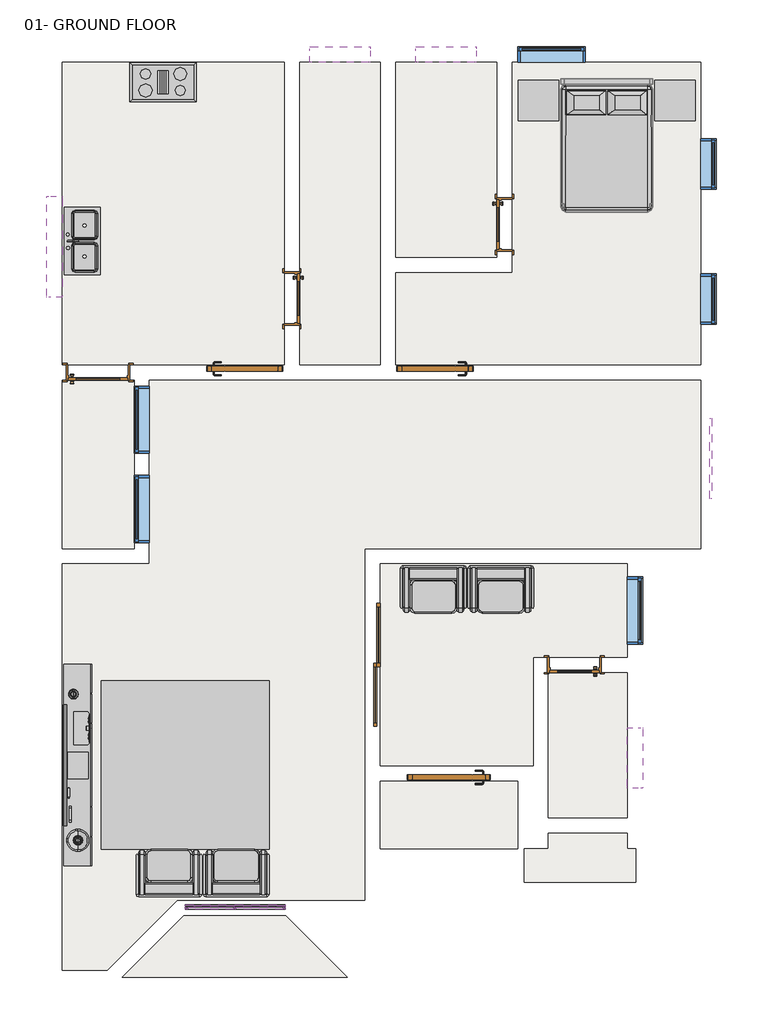
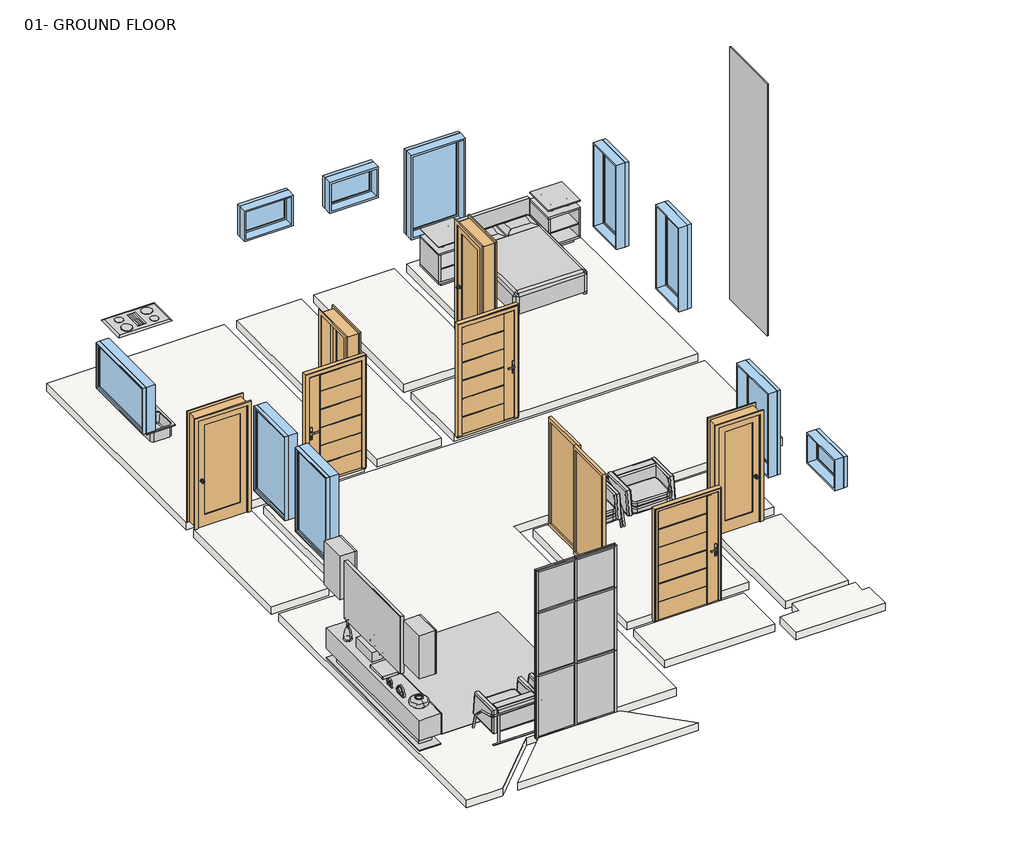
# One storey, incomplete: 17 members, 10 slabs, 10 windows, 9 furniture elements, 8 doors, 7 plates, 1 flow terminal, 1 proxy.
"""IFC4 building model written with IfcOpenShell, lengths in millimetres."""

from ifc_helpers import new_model, si_unit, frame, origin, place, context, project, spatial, polyline, outline, extrude, transform, mapped, element, save
from components import m_cook_top_4_unit_0915_x_500mm_6a9fc197, door_1104_x_2190_mm_4e9de5db, door_1104_x_2190_mm_38c8fb91, d1_d47119a4, m_door_interior_single_1_panel_wood_b1ec41f7, m_door_interior_single_1_panel_wood_1ba8bb0f, m_door_interior_single_1_panel_wood_d9b71ff8, sliding_2_panel_no_trim_2490c277, sink_kitchen_10_1000_x_535mm_bc591ed5, furniture_f593881e, furniture_82e6548d, furniture_15b88f3d, furniture_48082557, bed03_bed03_f6309305, bed_table_10474_bed_table_10474_77ad9a9a, bed_table_10474_bed_table_10474_76a96b03, couch_couch_04099933, rectangular_mullion_30mm_square_a2edb205, rectangular_mullion_30mm_square_7d0e1db8, rectangular_mullion_30mm_square_4c7eb74d, rectangular_mullion_30mm_square_e6372653, rectangular_mullion_30mm_square_88df2287, rectangular_mullion_30mm_square_3df302c3, rectangular_mullion_30mm_square_ca2f0e8b, rectangular_mullion_30mm_square_741b6552, system_panel_glazed_12388ada, system_panel_glazed_b614e8ed, system_panel_glazed_f246ada9, system_panel_glazed_70f3664f, system_panel_glazed_8799d416, m_fixed_w1_4c5c34d1, m_fixed_w2_a119b0d1, m_fixed_w3_kt_cae187e1, m_fixed_w4_tl_2657e552

model = new_model("IFC4")

# Units and contexts
model_context = context("Model", 3, world=origin())
ifc_project = project(units=[si_unit("LENGTHUNIT", "METRE", prefix="MILLI")], contexts=[model_context])

# Site, building, storey
site = spatial("IfcSite", under=ifc_project)
building = spatial("IfcBuilding", under=site)
storey = spatial("IfcBuildingStorey", under=building, Name="01- GROUND FLOOR", Elevation=450.0)

# Proxy
placement = place(None, origin())
m_cook_top_4_unit_0915_x_500mm_shape = m_cook_top_4_unit_0915_x_500mm_6a9fc197(model_context)
element("IfcBuildingElementProxy", 1, Name="M_Cook Top-4 Unit : 0915 x 500mm", ObjectType="M_Cook Top-4 Unit : 0915 x 500mm", at=placement, inside=storey, context=model_context, shape_type="MappedRepresentation", body=[
    mapped(m_cook_top_4_unit_0915_x_500mm_shape, transform((-8578.8712297, 3112.9985738, 450.0), x_axis=(1.0, 0.0, 0.0), y_axis=(0.0, 1.0, 0.0), z_axis=(0.0, 0.0, 1.0))),
])

# Doors
door_1104_x_2190_mm_shape = door_1104_x_2190_mm_4e9de5db(model_context)
element("IfcDoor", 2, ObjectType="1104 x 2190 mm", at=placement, inside=storey, context=model_context, shape_type="MappedRepresentation", body=[
    mapped(door_1104_x_2190_mm_shape, transform((-4533.8712297, -1202.0014262, 450.0), x_axis=(-1.0, 0.0, 0.0), y_axis=(0.0, -1.0, 0.0), z_axis=(0.0, 0.0, 1.0))),
])
door_1104_x_2190_mm_2_shape = door_1104_x_2190_mm_38c8fb91(model_context)
element("IfcDoor", 3, ObjectType="1104 x 2190 mm", at=placement, inside=storey, context=model_context, shape_type="MappedRepresentation", body=[
    mapped(door_1104_x_2190_mm_2_shape, transform((-7363.8712297, -1202.0014262, 450.0), x_axis=(1.0, 0.0, 0.0), y_axis=(0.0, 1.0, 0.0), z_axis=(0.0, 0.0, 1.0))),
])
d1_shape = d1_d47119a4(model_context)
element("IfcDoor", 4, ObjectType="D1", at=placement, inside=storey, context=model_context, shape_type="MappedRepresentation", body=[
    mapped(d1_shape, transform((-4328.8712297, -7162.0014262, 450.0), x_axis=(-1.0, 0.0, 0.0), y_axis=(0.0, -1.0, 0.0), z_axis=(0.0, 0.0, 1.0))),
])
m_door_interior_single_1_panel_wood_shape = m_door_interior_single_1_panel_wood_b1ec41f7(model_context)
element("IfcDoor", 5, ObjectType="M_Door-Interior-Single-1_Panel-Wood", at=placement, inside=storey, context=model_context, shape_type="MappedRepresentation", body=[
    mapped(m_door_interior_single_1_panel_wood_shape, transform((-9543.8712297, -1205.1764262, 450.0), x_axis=(1.0, 0.0, 0.0), y_axis=(0.0, 1.0, 0.0), z_axis=(0.0, 0.0, 1.0))),
])
m_door_interior_single_1_panel_wood_2_shape = m_door_interior_single_1_panel_wood_1ba8bb0f(model_context)
element("IfcDoor", 6, ObjectType="M_Door-Interior-Single-1_Panel-Wood", at=placement, inside=storey, context=model_context, shape_type="MappedRepresentation", body=[
    mapped(m_door_interior_single_1_panel_wood_2_shape, transform((-3507.0462297, 997.9985738, 450.0), x_axis=(0.0, -1.0, 0.0), y_axis=(1.0, 0.0, 0.0), z_axis=(0.0, 0.0, 1.0))),
])
m_door_interior_single_1_panel_wood_3_shape = m_door_interior_single_1_panel_wood_d9b71ff8(model_context)
element("IfcDoor", 7, ObjectType="M_Door-Interior-Single-1_Panel-Wood", at=placement, inside=storey, context=model_context, shape_type="MappedRepresentation", body=[
    mapped(m_door_interior_single_1_panel_wood_3_shape, transform((-6660.6962297, -102.0014262, 450.0), x_axis=(0.0, -1.0, 0.0), y_axis=(1.0, 0.0, 0.0), z_axis=(0.0, 0.0, 1.0))),
])
element("IfcDoor", 8, ObjectType="M_Door-Interior-Single-1_Panel-Wood", at=placement, inside=storey, context=model_context, shape_type="MappedRepresentation", body=[
    mapped(m_door_interior_single_1_panel_wood_3_shape, transform((-2463.8712297, -5550.1764262, 450.0), x_axis=(-1.0, 0.0, 0.0), y_axis=(0.0, -1.0, 0.0), z_axis=(0.0, 0.0, 1.0))),
])
sliding_2_panel_no_trim_shape = sliding_2_panel_no_trim_2490c277(model_context)
element("IfcDoor", 9, ObjectType="Sliding-2 panel_no trim", at=placement, inside=storey, context=model_context, shape_type="MappedRepresentation", body=[
    mapped(sliding_2_panel_no_trim_shape, transform((-5590.8712297, -5547.0014262, 900.0), x_axis=(0.0, -1.0, 0.0), y_axis=(1.0, 0.0, 0.0), z_axis=(0.0, 0.0, 1.0))),
])

# Flow terminal
sink_kitchen_10_1000_x_535mm_shape = sink_kitchen_10_1000_x_535mm_bc591ed5(model_context)
element("IfcFlowTerminal", 10, ObjectType="Sink - Kitchen (10) : 1000 x 535mm", at=placement, inside=storey, context=model_context, shape_type="MappedRepresentation", body=[
    mapped(sink_kitchen_10_1000_x_535mm_shape, transform((-9778.3258285, 735.4093333, 450.0), x_axis=(0.0, 1.0, 0.0), y_axis=(-1.0, 0.0, 0.0), z_axis=(0.0, 0.0, 1.0))),
])

# Furniture
furniture_shape = furniture_f593881e(model_context)
furniture_2_shape = furniture_82e6548d(model_context)
furniture_3_shape = furniture_15b88f3d(model_context)
element("IfcFurniture", 11, at=placement, inside=storey, context=model_context, shape_type="MappedRepresentation", body=[
    mapped(furniture_shape, transform((-10038.4053985, -7558.5028687, 450.0), x_axis=(0.0, 1.0, 0.0), y_axis=(-1.0, 0.0, 0.0), z_axis=(0.0, 0.0, 1.0))),
    mapped(furniture_2_shape, transform((-10038.4053985, -7558.5028687, 450.0), x_axis=(0.0, 1.0, 0.0), y_axis=(-1.0, 0.0, 0.0), z_axis=(0.0, 0.0, 1.0))),
    mapped(furniture_3_shape, transform((-10038.4053985, -7558.5028687, 450.0), x_axis=(0.0, 1.0, 0.0), y_axis=(-1.0, 0.0, 0.0), z_axis=(0.0, 0.0, 1.0))),
])
furniture_4_shape = furniture_48082557(model_context)
element("IfcFurniture", 12, at=placement, inside=storey, context=model_context, shape_type="MappedRepresentation", body=[
    mapped(furniture_4_shape, transform((-8248.3516855, -7033.5028687, 450.0), x_axis=(1.0, 0.0, 0.0), y_axis=(0.0, 1.0, 0.0), z_axis=(0.0, 0.0, 1.0))),
])
bed03_bed03_shape = bed03_bed03_f6309305(model_context)
element("IfcFurniture", 13, ObjectType="Bed03 : Bed03", at=placement, inside=storey, context=model_context, shape_type="MappedRepresentation", body=[
    mapped(bed03_bed03_shape, transform((-2667.6546586, 3162.5615242, 450.0), x_axis=(0.0, -1.0, 0.0), y_axis=(1.0, 0.0, 0.0), z_axis=(0.0, 0.0, 1.0))),
])
bed_table_10474_bed_table_10474_shape = bed_table_10474_bed_table_10474_77ad9a9a(model_context)
element("IfcFurniture", 14, ObjectType="Bed_Table_10474 : Bed_Table_10474", at=placement, inside=storey, context=model_context, shape_type="MappedRepresentation", body=[
    mapped(bed_table_10474_bed_table_10474_shape, transform((-967.6546586, 2842.5615242, 450.0), x_axis=(1.0, 0.0, 0.0), y_axis=(0.0, 1.0, 0.0), z_axis=(0.0, 0.0, 1.0))),
])
bed_table_10474_bed_table_10474_2_shape = bed_table_10474_bed_table_10474_76a96b03(model_context)
element("IfcFurniture", 15, ObjectType="Bed_Table_10474 : Bed_Table_10474", at=placement, inside=storey, context=model_context, shape_type="MappedRepresentation", body=[
    mapped(bed_table_10474_bed_table_10474_2_shape, transform((-2996.0546767, 2842.5615242, 450.0), x_axis=(-1.0, 0.0, 0.0), y_axis=(0.0, -1.0, 0.0), z_axis=(0.0, 0.0, 1.0))),
])
couch_couch_shape = couch_couch_04099933(model_context)
element("IfcFurniture", 16, ObjectType="Couch : Couch", at=placement, inside=storey, context=model_context, shape_type="MappedRepresentation", body=[
    mapped(couch_couch_shape, transform((-7488.3516855, -8533.5028687, 450.0), x_axis=(-1.0, 0.0, 0.0), y_axis=(0.0, -1.0, 0.0), z_axis=(0.0, 0.0, 1.0))),
])
element("IfcFurniture", 17, ObjectType="Couch : Couch", at=placement, inside=storey, context=model_context, shape_type="MappedRepresentation", body=[
    mapped(couch_couch_shape, transform((-8488.3516855, -8533.5028687, 450.0), x_axis=(-1.0, 0.0, 0.0), y_axis=(0.0, -1.0, 0.0), z_axis=(0.0, 0.0, 1.0))),
])
element("IfcFurniture", 18, ObjectType="Couch : Couch", at=placement, inside=storey, context=model_context, shape_type="MappedRepresentation", body=[
    mapped(couch_couch_shape, transform((-4558.8712297, -4532.0014262, 450.0), x_axis=(1.0, 0.0, 0.0), y_axis=(0.0, 1.0, 0.0), z_axis=(0.0, 0.0, 1.0))),
])
element("IfcFurniture", 19, ObjectType="Couch : Couch", at=placement, inside=storey, context=model_context, shape_type="MappedRepresentation", body=[
    mapped(couch_couch_shape, transform((-3558.8712297, -4532.0014262, 450.0), x_axis=(1.0, 0.0, 0.0), y_axis=(0.0, 1.0, 0.0), z_axis=(0.0, 0.0, 1.0))),
])

# Members
rectangular_mullion_30mm_square_shape = rectangular_mullion_30mm_square_a2edb205(model_context)
element("IfcMember", 20, ObjectType="Rectangular Mullion : 30mm Square", at=placement, inside=storey, context=model_context, shape_type="MappedRepresentation", body=[
    mapped(rectangular_mullion_30mm_square_shape, transform((-6793.8712297, -9162.0014262, 3750.0), x_axis=(0.0, 0.0, 1.0), y_axis=(0.0, -1.0, 0.0), z_axis=(1.0, 0.0, 0.0))),
])
element("IfcMember", 21, ObjectType="Rectangular Mullion : 30mm Square", at=placement, inside=storey, context=model_context, shape_type="MappedRepresentation", body=[
    mapped(rectangular_mullion_30mm_square_shape, transform((-7498.8712297, -9162.0014262, 450.0), x_axis=(0.0, 0.0, -1.0), y_axis=(0.0, -1.0, 0.0), z_axis=(-1.0, 0.0, 0.0))),
])
rectangular_mullion_30mm_square_2_shape = rectangular_mullion_30mm_square_7d0e1db8(model_context)
element("IfcMember", 22, ObjectType="Rectangular Mullion : 30mm Square", at=placement, inside=storey, context=model_context, shape_type="MappedRepresentation", body=[
    mapped(rectangular_mullion_30mm_square_2_shape, transform((-7513.8712297, -9162.0014262, 450.0), x_axis=(1.0, 0.0, 0.0), y_axis=(0.0, -1.0, 0.0), z_axis=(0.0, 0.0, -1.0))),
])
rectangular_mullion_30mm_square_3_shape = rectangular_mullion_30mm_square_4c7eb74d(model_context)
element("IfcMember", 23, ObjectType="Rectangular Mullion : 30mm Square", at=placement, inside=storey, context=model_context, shape_type="MappedRepresentation", body=[
    mapped(rectangular_mullion_30mm_square_3_shape, transform((-6793.8712297, -9162.0014262, 2925.0), x_axis=(0.0, 0.0, 1.0), y_axis=(0.0, -1.0, 0.0), z_axis=(1.0, 0.0, 0.0))),
])
element("IfcMember", 24, ObjectType="Rectangular Mullion : 30mm Square", at=placement, inside=storey, context=model_context, shape_type="MappedRepresentation", body=[
    mapped(rectangular_mullion_30mm_square_3_shape, transform((-6793.8712297, -9162.0014262, 1687.5), x_axis=(0.0, 0.0, 1.0), y_axis=(0.0, -1.0, 0.0), z_axis=(1.0, 0.0, 0.0))),
])
element("IfcMember", 25, ObjectType="Rectangular Mullion : 30mm Square", at=placement, inside=storey, context=model_context, shape_type="MappedRepresentation", body=[
    mapped(rectangular_mullion_30mm_square_2_shape, transform((-7513.8712297, -9162.0014262, 1687.5), x_axis=(1.0, 0.0, 0.0), y_axis=(0.0, -1.0, 0.0), z_axis=(0.0, 0.0, -1.0))),
])
rectangular_mullion_30mm_square_4_shape = rectangular_mullion_30mm_square_e6372653(model_context)
element("IfcMember", 26, ObjectType="Rectangular Mullion : 30mm Square", at=placement, inside=storey, context=model_context, shape_type="MappedRepresentation", body=[
    mapped(rectangular_mullion_30mm_square_4_shape, transform((-6763.8712297, -9162.0014262, 450.0), x_axis=(1.0, 0.0, 0.0), y_axis=(0.0, -1.0, 0.0), z_axis=(0.0, 0.0, -1.0))),
])
element("IfcMember", 27, ObjectType="Rectangular Mullion : 30mm Square", at=placement, inside=storey, context=model_context, shape_type="MappedRepresentation", body=[
    mapped(rectangular_mullion_30mm_square_4_shape, transform((-6763.8712297, -9162.0014262, 1687.5), x_axis=(1.0, 0.0, 0.0), y_axis=(0.0, -1.0, 0.0), z_axis=(0.0, 0.0, -1.0))),
])
element("IfcMember", 28, ObjectType="Rectangular Mullion : 30mm Square", at=placement, inside=storey, context=model_context, shape_type="MappedRepresentation", body=[
    mapped(rectangular_mullion_30mm_square_4_shape, transform((-8243.8712297, -9162.0014262, 2925.0), x_axis=(-1.0, 0.0, 0.0), y_axis=(0.0, -1.0, 0.0), z_axis=(0.0, 0.0, 1.0))),
])
element("IfcMember", 29, ObjectType="Rectangular Mullion : 30mm Square", at=placement, inside=storey, context=model_context, shape_type="MappedRepresentation", body=[
    mapped(rectangular_mullion_30mm_square_4_shape, transform((-8243.8712297, -9162.0014262, 1687.5), x_axis=(-1.0, 0.0, 0.0), y_axis=(0.0, -1.0, 0.0), z_axis=(0.0, 0.0, 1.0))),
])
rectangular_mullion_30mm_square_5_shape = rectangular_mullion_30mm_square_88df2287(model_context)
element("IfcMember", 30, ObjectType="Rectangular Mullion : 30mm Square", at=placement, inside=storey, context=model_context, shape_type="MappedRepresentation", body=[
    mapped(rectangular_mullion_30mm_square_5_shape, transform((-8213.8712297, -9162.0014262, 450.0), x_axis=(0.0, 0.0, -1.0), y_axis=(0.0, -1.0, 0.0), z_axis=(-1.0, 0.0, 0.0))),
])
rectangular_mullion_30mm_square_6_shape = rectangular_mullion_30mm_square_3df302c3(model_context)
element("IfcMember", 31, ObjectType="Rectangular Mullion : 30mm Square", at=placement, inside=storey, context=model_context, shape_type="MappedRepresentation", body=[
    mapped(rectangular_mullion_30mm_square_6_shape, transform((-7528.8712297, -9162.0014262, 2925.0), x_axis=(0.0, 0.0, 1.0), y_axis=(0.0, -1.0, 0.0), z_axis=(1.0, 0.0, 0.0))),
])
element("IfcMember", 32, ObjectType="Rectangular Mullion : 30mm Square", at=placement, inside=storey, context=model_context, shape_type="MappedRepresentation", body=[
    mapped(rectangular_mullion_30mm_square_6_shape, transform((-7528.8712297, -9162.0014262, 1687.5), x_axis=(0.0, 0.0, 1.0), y_axis=(0.0, -1.0, 0.0), z_axis=(1.0, 0.0, 0.0))),
])
element("IfcMember", 33, ObjectType="Rectangular Mullion : 30mm Square", at=placement, inside=storey, context=model_context, shape_type="MappedRepresentation", body=[
    mapped(rectangular_mullion_30mm_square_5_shape, transform((-7528.8712297, -9162.0014262, 3750.0), x_axis=(0.0, 0.0, 1.0), y_axis=(0.0, -1.0, 0.0), z_axis=(1.0, 0.0, 0.0))),
])
rectangular_mullion_30mm_square_7_shape = rectangular_mullion_30mm_square_ca2f0e8b(model_context)
element("IfcMember", 34, ObjectType="Rectangular Mullion : 30mm Square", at=placement, inside=storey, context=model_context, shape_type="MappedRepresentation", body=[
    mapped(rectangular_mullion_30mm_square_7_shape, transform((-7513.8712297, -9162.0014262, 2925.0), x_axis=(1.0, 0.0, 0.0), y_axis=(0.0, -1.0, 0.0), z_axis=(0.0, 0.0, -1.0))),
])
rectangular_mullion_30mm_square_8_shape = rectangular_mullion_30mm_square_741b6552(model_context)
element("IfcMember", 35, ObjectType="Rectangular Mullion : 30mm Square", at=placement, inside=storey, context=model_context, shape_type="MappedRepresentation", body=[
    mapped(rectangular_mullion_30mm_square_8_shape, transform((-8243.8712297, -9162.0014262, 3750.0), x_axis=(-1.0, 0.0, 0.0), y_axis=(0.0, -1.0, 0.0), z_axis=(0.0, 0.0, 1.0))),
])
element("IfcMember", 36, ObjectType="Rectangular Mullion : 30mm Square", at=placement, inside=storey, context=model_context, shape_type="MappedRepresentation", body=[
    mapped(rectangular_mullion_30mm_square_8_shape, transform((-6763.8712297, -9162.0014262, 2925.0), x_axis=(1.0, 0.0, 0.0), y_axis=(0.0, -1.0, 0.0), z_axis=(0.0, 0.0, -1.0))),
])

# Plates
system_panel_glazed_shape = system_panel_glazed_12388ada(model_context)
element("IfcPlate", 37, ObjectType="System Panel : Glazed", at=placement, inside=storey, context=model_context, shape_type="MappedRepresentation", body=[
    mapped(system_panel_glazed_shape, transform((-7138.8712297, -9162.0014262, 450.0), x_axis=(1.0, 0.0, 0.0), y_axis=(0.0, 1.0, 0.0), z_axis=(0.0, 0.0, 1.0))),
])
element("IfcPlate", 38, ObjectType="System Panel : Glazed", at=placement, inside=storey, context=model_context, shape_type="MappedRepresentation", body=[
    mapped(system_panel_glazed_shape, transform((-7138.8712297, -9162.0014262, 1687.5), x_axis=(1.0, 0.0, 0.0), y_axis=(0.0, 1.0, 0.0), z_axis=(0.0, 0.0, 1.0))),
])
system_panel_glazed_2_shape = system_panel_glazed_b614e8ed(model_context)
element("IfcPlate", 39, ObjectType="System Panel : Glazed", at=placement, inside=storey, context=model_context, shape_type="MappedRepresentation", body=[
    mapped(system_panel_glazed_2_shape, transform((-7878.8712297, -9162.0014262, 450.0), x_axis=(1.0, 0.0, 0.0), y_axis=(0.0, 1.0, 0.0), z_axis=(0.0, 0.0, 1.0))),
])
element("IfcPlate", 40, ObjectType="System Panel : Glazed", at=placement, inside=storey, context=model_context, shape_type="MappedRepresentation", body=[
    mapped(system_panel_glazed_2_shape, transform((-7878.8712297, -9162.0014262, 1687.5), x_axis=(1.0, 0.0, 0.0), y_axis=(0.0, 1.0, 0.0), z_axis=(0.0, 0.0, 1.0))),
])
system_panel_glazed_3_shape = system_panel_glazed_f246ada9(model_context)
element("IfcPlate", 41, ObjectType="System Panel : Glazed", at=placement, inside=storey, context=model_context, shape_type="MappedRepresentation", body=[
    mapped(system_panel_glazed_3_shape, transform((-7878.8712297, -9162.0014262, 2925.0), x_axis=(1.0, 0.0, 0.0), y_axis=(0.0, 1.0, 0.0), z_axis=(0.0, 0.0, 1.0))),
])
system_panel_glazed_4_shape = system_panel_glazed_70f3664f(model_context)
element("IfcPlate", 42, ObjectType="System Panel : Glazed", at=placement, inside=storey, context=model_context, shape_type="MappedRepresentation", body=[
    mapped(system_panel_glazed_4_shape, transform((-7138.8712297, -9162.0014262, 2925.0), x_axis=(1.0, 0.0, 0.0), y_axis=(0.0, 1.0, 0.0), z_axis=(0.0, 0.0, 1.0))),
])
system_panel_glazed_5_shape = system_panel_glazed_8799d416(model_context)
element("IfcPlate", 43, ObjectType="System Panel : Glazed", at=placement, inside=storey, context=model_context, shape_type="MappedRepresentation", body=[
    mapped(system_panel_glazed_5_shape, transform((-473.8712297, -2480.571442, 1950.0), x_axis=(0.0, -1.0, 0.0), y_axis=(1.0, 0.0, 0.0), z_axis=(0.0, 0.0, 1.0))),
])

# Slabs
element("IfcSlab", 44, ObjectType="150", at=placement, inside=storey, context=model_context, shape_type="SweptSolid", body=[
    extrude(outline(polyline([(-6778.8712297, -1087.0014262), (-10078.8712297, -1087.0014262), (-10078.8712297, 3412.9985738), (-6778.8712297, 3412.9985738), (-6778.8712297, -1087.0014262)])), frame((0.0, 0.0, 300.0), z_axis=(0.0, 0.0, 1.0), x_axis=(1.0, 0.0, 0.0)), (0.0, 0.0, 1.0), 150.0),
])
element("IfcSlab", 45, ObjectType="150", at=placement, inside=storey, context=model_context, shape_type="SweptSolid", body=[
    extrude(outline(polyline([(-5348.8712297, 3412.9985738), (-5348.8712297, -1087.0014262), (-6548.8712297, -1087.0014262), (-6548.8712297, 3412.9985738), (-5348.8712297, 3412.9985738)])), frame((0.0, 0.0, 300.0), z_axis=(0.0, 0.0, 1.0), x_axis=(1.0, 0.0, 0.0)), (0.0, 0.0, 1.0), 150.0),
])
element("IfcSlab", 46, ObjectType="150", at=placement, inside=storey, context=model_context, shape_type="SweptSolid", body=[
    extrude(outline(polyline([(-3618.8712297, 3412.9985738), (-3618.8712297, 512.9985738), (-5118.8712297, 512.9985738), (-5118.8712297, 3412.9985738), (-3618.8712297, 3412.9985738)])), frame((0.0, 0.0, 300.0), z_axis=(0.0, 0.0, 1.0), x_axis=(1.0, 0.0, 0.0)), (0.0, 0.0, 1.0), 150.0),
])
element("IfcSlab", 47, ObjectType="150", at=placement, inside=storey, context=model_context, shape_type="SweptSolid", body=[
    extrude(outline(polyline([(-9008.8712297, -3817.0014262), (-10078.8712297, -3817.0014262), (-10078.8712297, -1317.0014262), (-9008.8712297, -1317.0014262), (-9008.8712297, -3817.0014262)])), frame((0.0, 0.0, 300.0), z_axis=(0.0, 0.0, 1.0), x_axis=(1.0, 0.0, 0.0)), (0.0, 0.0, 1.0), 150.0),
])
element("IfcSlab", 48, ObjectType="150", at=placement, inside=storey, context=model_context, shape_type="SweptSolid", body=[
    extrude(outline(polyline([(-1678.8712297, -5662.0014262), (-1678.8712297, -7817.0014262), (-2848.8712297, -7817.0014262), (-2848.8712297, -5662.0014262), (-1678.8712297, -5662.0014262)])), frame((0.0, 0.0, 300.0), z_axis=(0.0, 0.0, 1.0), x_axis=(1.0, 0.0, 0.0)), (0.0, 0.0, 1.0), 150.0),
])
element("IfcSlab", 49, ObjectType="150", at=placement, inside=storey, context=model_context, shape_type="SweptSolid", body=[
    extrude(outline(polyline([(-1678.8712297, -4047.0014262), (-1678.8712297, -5432.0014262), (-3078.8712297, -5432.0014262), (-3078.8712297, -7047.0014262), (-5348.8712297, -7047.0014262), (-5348.8712297, -4047.0014262), (-1678.8712297, -4047.0014262)])), frame((0.0, 0.0, 300.0), z_axis=(0.0, 0.0, 1.0), x_axis=(1.0, 0.0, 0.0)), (0.0, 0.0, 1.0), 150.0),
])
element("IfcSlab", 50, ObjectType="150", at=placement, inside=storey, context=model_context, shape_type="SweptSolid", body=[
    extrude(outline(polyline([(-5578.8712297, -9047.0014262), (-8363.4139709, -9047.0014262), (-9403.4139709, -10087.0014262), (-10078.8712297, -10087.0014262), (-10078.8712297, -4047.0014262), (-8778.8712297, -4047.0014262), (-8778.8712297, -1317.0014262), (-588.8712297, -1317.0014262), (-588.8712297, -3817.0014262), (-5578.8712297, -3817.0014262), (-5578.8712297, -9047.0014262)])), frame((0.0, 0.0, 300.0), z_axis=(0.0, 0.0, 1.0), x_axis=(1.0, 0.0, 0.0)), (0.0, 0.0, 1.0), 150.0),
])
element("IfcSlab", 51, ObjectType="150", at=placement, inside=storey, context=model_context, shape_type="SweptSolid", body=[
    extrude(outline(polyline([(-5118.8712297, -1087.0014262), (-5118.8712297, 282.9985738), (-3388.8712297, 282.9985738), (-3388.8712297, 3412.9985738), (-588.8712297, 3412.9985738), (-588.8712297, -1087.0014262), (-5118.8712297, -1087.0014262)])), frame((0.0, 0.0, 300.0), z_axis=(0.0, 0.0, 1.0), x_axis=(1.0, 0.0, 0.0)), (0.0, 0.0, 1.0), 150.0),
])
element("IfcSlab", 52, ObjectType="150", at=placement, inside=storey, context=model_context, shape_type="SweptSolid", body=[
    extrude(outline(polyline([(-3308.8712297, -7277.0014262), (-3308.8712297, -8277.0014262), (-5348.8712297, -8277.0014262), (-5348.8712297, -7277.0014262), (-3308.8712297, -7277.0014262)])), frame((0.0, 0.0, 300.0), z_axis=(0.0, 0.0, 1.0), x_axis=(1.0, 0.0, 0.0)), (0.0, 0.0, 1.0), 150.0),
])
element("IfcSlab", 53, ObjectType="150", at=placement, inside=storey, context=model_context, shape_type="SweptSolid", body=[
    extrude(outline(polyline([(-8268.1448516, -9277.0014262), (-6751.5057893, -9277.0014262), (-5836.5057893, -10192.0014262), (-9183.1448516, -10192.0014262), (-8268.1448516, -9277.0014262)])), frame((0.0, 0.0, 400.0), z_axis=(0.0, 0.0, 1.0), x_axis=(1.0, 0.0, 0.0)), (0.0, 0.0, 1.0), 150.0),
    extrude(outline(polyline([(-3208.8712297, -8277.0014262), (-2848.8712297, -8277.0014262), (-2848.8712297, -8047.0014262), (-1678.8712297, -8047.0014262), (-1678.8712297, -8277.0014262), (-1548.8712297, -8277.0014262), (-1548.8712297, -8777.0014262), (-3208.8712297, -8777.0014262), (-3208.8712297, -8277.0014262)])), frame((0.0, 0.0, 400.0), z_axis=(0.0, 0.0, 1.0), x_axis=(1.0, 0.0, 0.0)), (0.0, 0.0, 1.0), 150.0),
])

# Windows
m_fixed_w1_shape = m_fixed_w1_4c5c34d1(model_context)
element("IfcWindow", 54, ObjectType="M_Fixed : W1", at=placement, inside=storey, context=model_context, shape_type="MappedRepresentation", body=[
    mapped(m_fixed_w1_shape, transform((-2803.8712297, 3514.9985738, 450.0), x_axis=(1.0, 0.0, 0.0), y_axis=(0.0, 1.0, 0.0), z_axis=(0.0, 0.0, 1.0))),
])
element("IfcWindow", 55, ObjectType="M_Fixed : W1", at=placement, inside=storey, context=model_context, shape_type="MappedRepresentation", body=[
    mapped(m_fixed_w1_shape, transform((-1576.8712297, -4739.5014262, 450.0), x_axis=(0.0, -1.0, 0.0), y_axis=(1.0, 0.0, 0.0), z_axis=(0.0, 0.0, 1.0))),
])
element("IfcWindow", 56, ObjectType="M_Fixed : W1", at=placement, inside=storey, context=model_context, shape_type="MappedRepresentation", body=[
    mapped(m_fixed_w1_shape, transform((-8880.8712297, -1902.0014262, 450.0), x_axis=(0.0, 1.0, 0.0), y_axis=(-1.0, 0.0, 0.0), z_axis=(0.0, 0.0, 1.0))),
])
element("IfcWindow", 57, ObjectType="M_Fixed : W1", at=placement, inside=storey, context=model_context, shape_type="MappedRepresentation", body=[
    mapped(m_fixed_w1_shape, transform((-8880.8712297, -3232.0014262, 450.0), x_axis=(0.0, 1.0, 0.0), y_axis=(-1.0, 0.0, 0.0), z_axis=(0.0, 0.0, 1.0))),
])
m_fixed_w2_shape = m_fixed_w2_a119b0d1(model_context)
element("IfcWindow", 58, ObjectType="M_Fixed : W2", at=placement, inside=storey, context=model_context, shape_type="MappedRepresentation", body=[
    mapped(m_fixed_w2_shape, transform((-486.8712297, 1897.9985738, 450.0), x_axis=(0.0, -1.0, 0.0), y_axis=(1.0, 0.0, 0.0), z_axis=(0.0, 0.0, 1.0))),
])
element("IfcWindow", 59, ObjectType="M_Fixed : W2", at=placement, inside=storey, context=model_context, shape_type="MappedRepresentation", body=[
    mapped(m_fixed_w2_shape, transform((-486.8712297, -112.0014262, 450.0), x_axis=(0.0, -1.0, 0.0), y_axis=(1.0, 0.0, 0.0), z_axis=(0.0, 0.0, 1.0))),
])
m_fixed_w3_kt_shape = m_fixed_w3_kt_cae187e1(model_context)
element("IfcWindow", 60, ObjectType="M_Fixed : W3 KT", at=placement, inside=storey, context=model_context, shape_type="MappedRepresentation", body=[
    mapped(m_fixed_w3_kt_shape, transform((-10180.8712297, 667.9985738, 450.0), x_axis=(0.0, 1.0, 0.0), y_axis=(-1.0, 0.0, 0.0), z_axis=(0.0, 0.0, 1.0))),
])
m_fixed_w4_tl_shape = m_fixed_w4_tl_2657e552(model_context)
element("IfcWindow", 61, ObjectType="M_Fixed : W4 TL", at=placement, inside=storey, context=model_context, shape_type="MappedRepresentation", body=[
    mapped(m_fixed_w4_tl_shape, transform((-5948.8712297, 3514.9985738, 450.0), x_axis=(1.0, 0.0, 0.0), y_axis=(0.0, 1.0, 0.0), z_axis=(0.0, 0.0, 1.0))),
])
element("IfcWindow", 62, ObjectType="M_Fixed : W4 TL", at=placement, inside=storey, context=model_context, shape_type="MappedRepresentation", body=[
    mapped(m_fixed_w4_tl_shape, transform((-4368.8712297, 3514.9985738, 450.0), x_axis=(1.0, 0.0, 0.0), y_axis=(0.0, 1.0, 0.0), z_axis=(0.0, 0.0, 1.0))),
])
element("IfcWindow", 63, ObjectType="M_Fixed : W4 TL", at=placement, inside=storey, context=model_context, shape_type="MappedRepresentation", body=[
    mapped(m_fixed_w4_tl_shape, transform((-1576.8712297, -6932.0014262, 450.0), x_axis=(0.0, -1.0, 0.0), y_axis=(1.0, 0.0, 0.0), z_axis=(0.0, 0.0, 1.0))),
])

save(model, "model.ifc")

# Revit data of these elements
# Type "M_Cook Top-4 Unit : 0915 x 500mm"
#   Counter Height = 900 mm
#   Depth = 500 mm
#   Width = 915 mm
#   Burner Material = Metal - Chrome
#   Cooktop Material = Metal - Steel, Polished
#   Default Elevation = 0
# Type "1104 x 2190 mm"
#   Type Mark = "28"
#   Water resistance = "up to Class E900, EN 12208:2001"
#   Uniclass2015Version = "v1.21"
#   Uniclass2015Reference = "Ss_25_30_20_30"
#   Uniclass2015Description = "Frame and door leaf system"
#   URL = "www.aluprof.eu"
#   Type IFC Predefined Type = "USERDEFINED"
#   Right-hand / Left-hand door [instance default] = ""
#   Resistance to wind load = "up to Class C5/B5, EN 12210:2001"
#   Insert type = "ST"
#   Hardware [instance default] = ""
#   Product page = "https://aluprof.eu/en/architects/offer/window-and-door-systems/panel-doors#visualisation"
#   Operation = "SinglePanelOutwardOpening"
#   Opening type = "Outward"
#   NBSReference = "25-50-20/125"
#   NBSDescription = "Frame and door leaf system"
#   Important = "The actual acceptable construction dimensions are dependent on the selection of profiles and hardware, glazing type, construction weight and the construction’s operating conditions. These should be determined by a suitably qualified person, and using ALUPROF’s calculation software"
#   IfcExportType = "USERDEFINED"
#   IfcExportAs = "IfcDoorType"
#   Handle type [instance default] = ""
#   Manufacturer = "ALUPROF"
#   Export Type to IFC As = "IfcDoorType"
#   Door sill type [instance default] = ""
#   Description = "External single-leaf panel door outward opening"
#   Model = "MB-86 ST Panel Door AD07"
#   Content of the recyclate in the material = "69.2"
#   COBie.Type.WarrantyDurationParts = ""
#   COBie.Type.Name = ""
#   COBie.Type.Manufacturer = "ALUPROF S.A."
#   COBie.Space.Name = ""
#   COBie.Floor.Name = ""
#   COBie.Facility.Name = ""
#   COBie.CreatedOn = ""
#   COBie.Component.WarrantyStartDate = ""
#   COBie.Component.Name = "MB-86 ST Panel Door AD07"
#   Burglar resistance = "RC2"
#   Air permeability = "up to Class 4, EN 12207:2001"
#   Width of the active leaf = 1007.4 mm
#   Placement in wall = 20 mm
#   Thickness = 77 mm
#   Height of the opening sash = 2124.5 mm
#   Handle Offset = 1050 mm
#   Glazing thickness = 48 mm
#   Rough Height = 2250.7 mm
#   Rough Width = 1134.5 mm
#   Height = 2189.5 mm
#   Width = 1104.5 mm
#   Construction depth = 77 mm
#   Clear opening width = 900 mm
#   Clear opening height = 2100 mm
#   Height of the array = 341.583 mm
#   Schedule No. [instance default] = 1
#   Handrail = no
#   IsExternal = yes
#   Handle = yes
#   Door closer [instance default] = no
#   Function = 1
#   COBie.Type = yes
#   COBie = yes
#   Access control [instance default] = no
#   Panel = element 260956
#   Wall Closure = (empty or 0)
# Type "D1"
#   Type Mark = "22"
#   Water resistance = "up to Class E900, EN 12208:2001"
#   Uniclass2015Version = "v1.21"
#   Uniclass2015Reference = "Ss_25_30_20_30"
#   Uniclass2015Description = "Frame and door leaf system"
#   URL = "www.aluprof.eu"
#   Type IFC Predefined Type = "USERDEFINED"
#   Right-hand / Left-hand door [instance default] = ""
#   Resistance to wind load = "up to Class C5/B5, EN 12210:2001"
#   Insert type = "ST"
#   Hardware [instance default] = ""
#   Product page = "https://aluprof.eu/en/architects/offer/window-and-door-systems/panel-doors#visualisation"
#   Operation = "SinglePanelOutwardOpening"
#   Opening type = "Outward"
#   NBSReference = "25-50-20/125"
#   NBSDescription = "Frame and door leaf system"
#   Important = "The actual acceptable construction dimensions are dependent on the selection of profiles and hardware, glazing type, construction weight and the construction’s operating conditions. These should be determined by a suitably qualified person, and using ALUPROF’s calculation software"
#   IfcExportType = "USERDEFINED"
#   IfcExportAs = "IfcDoorType"
#   Handle type [instance default] = ""
#   Manufacturer = "ALUPROF"
#   Export Type to IFC As = "IfcDoorType"
#   Door sill type [instance default] = ""
#   Description = "External single-leaf panel door outward opening"
#   Model = "MB-86 ST Panel Door AD07"
#   Content of the recyclate in the material = "69.2"
#   COBie.Type.WarrantyDurationParts = ""
#   COBie.Type.Name = ""
#   COBie.Type.Manufacturer = "ALUPROF S.A."
#   COBie.Space.Name = ""
#   COBie.Floor.Name = ""
#   COBie.Facility.Name = ""
#   COBie.CreatedOn = ""
#   COBie.Component.WarrantyStartDate = ""
#   COBie.Component.Name = "MB-86 ST Panel Door AD07"
#   Burglar resistance = "RC2"
#   Air permeability = "up to Class 4, EN 12207:2001"
#   Width of the active leaf = 1107.4 mm
#   Placement in wall = 20 mm
#   Thickness = 77 mm
#   Height of the opening sash = 2124.5 mm
#   Handle Offset = 1050 mm
#   Glazing thickness = 48 mm
#   Rough Height = 2250.7 mm
#   Rough Width = 1234.5 mm
#   Height = 2189.5 mm
#   Width = 1204.5 mm
#   Construction depth = 77 mm
#   Clear opening width = 1000 mm
#   Clear opening height = 2100 mm
#   Height of the array = 341.583 mm
#   Schedule No. [instance default] = 1
#   Handrail = no
#   IsExternal = yes
#   Handle = yes
#   Door closer [instance default] = no
#   Function = 1
#   COBie.Type = yes
#   COBie = yes
#   Access control [instance default] = no
#   Panel = element 260956
#   Wall Closure = (empty or 0)
# Type "M_Door-Interior-Single-1_Panel-Wood"
#   Type Mark = "26"
#   Assembly Code = "C1020300"
#   Analytic Construction = "Wooden"
#   Top Rail = 120 mm
#   Thickness = 35 mm
#   Thermal Resistance (R) = 0.455703 (m²·K)/W
#   Swing Angle [instance default] = 90.00°
#   Stiles = 120 mm
#   Rough Width = 950 mm
#   Rough Height = 2125 mm
#   Height = 2100 mm
#   Width = 900 mm
#   Heat Transfer Coefficient (U) = 2.19465 W/(m²·K)
#   Bottom Rail = 230 mm
#   Trim Material = Cherry
#   Panel Material = Cherry
#   Frame Material = Cherry
#   Door Handle Material = Aluminum
#   Visual Light Transmittance = 0
#   Solar Heat Gain Coefficient = 0
#   Wall Closure = (empty or 0)
#   Function = (empty or 0)
# Type "M_Door-Interior-Single-1_Panel-Wood"
#   Type Mark = "23"
#   Assembly Code = "C1020300"
#   Analytic Construction = "Wooden"
#   Top Rail = 120 mm
#   Thickness = 35 mm
#   Thermal Resistance (R) = 0.455703 (m²·K)/W
#   Swing Angle [instance default] = 90.00°
#   Stiles = 120 mm
#   Rough Width = 800 mm
#   Rough Height = 2125 mm
#   Height = 2100 mm
#   Width = 750 mm
#   Heat Transfer Coefficient (U) = 2.19465 W/(m²·K)
#   Bottom Rail = 230 mm
#   Trim Material = Cherry
#   Panel Material = Cherry
#   Frame Material = Cherry
#   Door Handle Material = Aluminum
#   Visual Light Transmittance = 0
#   Solar Heat Gain Coefficient = 0
#   Wall Closure = (empty or 0)
#   Function = (empty or 0)
# Type "Sliding-2 panel_no trim"
#   Type Mark = "45"
#   Thickness = 50.006 mm
#   Height = 2133.997 mm
#   Rail Width = 75.009 mm
#   Stile Width = 50.006 mm
#   Width = 1829.991 mm
#   Door Material = Door - Panel
#   Frame Material = Door - Frame
#   Function = (empty or 0)
#   Assembly Code = ""
#   Wall Closure = (empty or 0)
# Type "Sink - Kitchen (10) : 1000 x 535mm"
#   Keynote = "N13/180"
#   Counter Height = 900 mm
#   Depth = 535 mm
#   Width = 1000 mm
#   Fixture Material = Metal - Stainless Steel, Polished
#   Sink Material = Metal - Stainless Steel, Polished
#   Default Elevation = 0
# Type
#   Default Elevation = 0
# Type
#   Width - Anchura = 2500 mm
#   Thickness - Espesor = 10 mm
#   Large - Largo = 2500 mm
#   Default Elevation = 1219.2 mm
# Type "Bed03 : Bed03"
#   Default Elevation = 0
# Type "Bed_Table_10474 : Bed_Table_10474"
#   myf = ""
#   Default Elevation = 0
# Type "Couch : Couch"
#   Fabric = Blue leather
#   Default Elevation = 0
#   Assembly Code = ""
# Type "Rectangular Mullion : 30mm Square"
#   built-in parameter 1007304 = 0.0984252 (stored number, unit not read)
#   built-in parameter 1007301 = 0.0492126 (stored number, unit not read)
#   built-in parameter 1007300 = 0.0492126 (stored number, unit not read)
# Type "150"
#   Function = 0
#   Layers, outside or top first: 150 mm "J FLOOR" (function 1)
# Type "M_Fixed : W1"
#   Type Mark = "19"
#   Height = 1650 mm
#   Default Sill Height = 450 mm
#   Width = 1000 mm
#   Window Inset = 19 mm
#   Frame Exterior Material = Iron, Ductile
#   Frame Interior Material = Iron, Ductile
#   Glass Pane Material = Glass
#   Sash = Iron, Ductile
#   Wall Closure = (empty or 0)
# Type "M_Fixed : W2"
#   Type Mark = "20"
#   Height = 1650 mm
#   Default Sill Height = 450 mm
#   Width = 750 mm
#   Window Inset = 19 mm
#   Frame Exterior Material = Iron, Ductile
#   Frame Interior Material = Iron, Ductile
#   Glass Pane Material = Glass
#   Sash = Iron, Ductile
#   Wall Closure = (empty or 0)
# Type "M_Fixed : W3 KT"
#   Type Mark = "21"
#   Height = 900 mm
#   Default Sill Height = 1200 mm
#   Width = 1500 mm
#   Window Inset = 19 mm
#   Frame Exterior Material = Iron, Ductile
#   Frame Interior Material = Iron, Ductile
#   Glass Pane Material = Glass
#   Sash = Iron, Ductile
#   Wall Closure = (empty or 0)
# Type "M_Fixed : W4 TL"
#   Type Mark = "22"
#   Height = 600 mm
#   Default Sill Height = 1500 mm
#   Width = 900 mm
#   Window Inset = 19 mm
#   Frame Exterior Material = Iron, Ductile
#   Frame Interior Material = Iron, Ductile
#   Glass Pane Material = Glass
#   Sash = Iron, Ductile
#   Wall Closure = (empty or 0)
# Element 1 (IfcBuildingElementProxy, "M_Cook Top-4 Unit : 0915 x 500mm")
#   Phase Created = New Construction
#   Materials on its faces: "Metal - Chrome", "Metal - Steel, Polished"
# Elements 2, 3 (IfcDoor, "1104 x 2190 mm")
#   Right-hand / Left-hand door = ""
#   Hardware = ""
#   Handle type = ""
#   Door sill type = ""
#   Schedule No. = 1
#   Door closer = no
#   Access control = no
#   Phase Created = New Construction
# Element 4 (IfcDoor, "D1")
#   Right-hand / Left-hand door = ""
#   Hardware = ""
#   Handle type = ""
#   Door sill type = ""
#   Schedule No. = 1
#   Door closer = no
#   Access control = no
#   Phase Created = New Construction
# Elements 5, 6, 7, 8 (IfcDoor, "M_Door-Interior-Single-1_Panel-Wood")
#   Swing Angle = 90.00°
#   Phase Created = New Construction
#   Materials on its faces: "Cherry", "Aluminum"
# Element 9 (IfcDoor, "Sliding-2 panel_no trim")
#   Phase Created = New Construction
#   Materials on its faces: "Door - Panel", "Glass"
# Element 10 (IfcFlowTerminal, "Sink - Kitchen (10) : 1000 x 535mm")
#   Mark = "1"
#   Phase Created = New Construction
#   Materials on its faces: "Metal - Stainless Steel, Polished"
# Element 11 (IfcFurniture)
#   Phase Created = New Construction
#   Materials on its faces: "Phase - Demo", "wood 2(1)", "Porcelain, Ivory", "silver", "lit", "Default(1)", "Default Wall", "light", "wood 2", "tv button", "Modern Cabinet", "tv body", "Default", "Poche(1)", "Base Material", "Glass", "gold", "Sculpture"
# Element 12 (IfcFurniture)
#   Phase Created = New Construction
# Element 13 (IfcFurniture, "Bed03 : Bed03")
#   Phase Created = New Construction
# Elements 14, 15 (IfcFurniture, "Bed_Table_10474 : Bed_Table_10474")
#   Phase Created = New Construction
#   Materials on its faces: "metal table", "madera", "glass table"
# Elements 16, 17, 18, 19 (IfcFurniture, "Couch : Couch")
#   Phase Created = New Construction
#   Materials on its faces: "Blue leather"
# Elements 20, 21, 22, 23, 24, 25, 26, 27, 28, 29, 30, 31, 32, 33, 34, 35, 36 (IfcMember, "Rectangular Mullion : 30mm Square")
#   Phase Created = New Construction
#   Materials on its faces: "Aluminum"
# Elements 37, 38, 39, 40, 41, 42, 43 (IfcPlate, "System Panel : Glazed")
#   Phase Created = New Construction
#   Materials on its faces: "Glass"
# Elements 44, 45 (IfcSlab, "150")
#   Height Offset From Level = 0 mm
#   Phase Created = New Construction
#   Materials on its faces: "J FLOOR", "Tiles 22"
# Elements 46, 48 (IfcSlab, "150")
#   Height Offset From Level = 0 mm
#   Phase Created = New Construction
#   Materials on its faces: "J FLOOR", "Tiles 13"
# Elements 47, 49, 52 (IfcSlab, "150")
#   Height Offset From Level = 0 mm
#   Phase Created = New Construction
#   Materials on its faces: "J FLOOR", "Marble 06"
# Element 50 (IfcSlab, "150")
#   built-in parameter 1001955 = -1.5708 (stored number, unit not read)
#   Height Offset From Level = 0 mm
#   Phase Created = New Construction
#   Materials on its faces: "J FLOOR", "Marble 05"
# Element 51 (IfcSlab, "150")
#   built-in parameter 1001955 = 3.14159 (stored number, unit not read)
#   Height Offset From Level = 0 mm
#   Phase Created = New Construction
#   Materials on its faces: "J FLOOR"
# Element 53 (IfcSlab, "150")
#   built-in parameter 1001955 = 0.785398 (stored number, unit not read)
#   Height Offset From Level = 100 mm
#   Phase Created = New Construction
#   Materials on its faces: "J FLOOR", "Grass 01"
# Element 54 (IfcWindow, "M_Fixed : W1")
#   Mark = "6"
#   Phase Created = New Construction
#   Materials on its faces: "Iron, Ductile", "Glass"
# Element 55 (IfcWindow, "M_Fixed : W1")
#   Mark = "13"
#   Phase Created = New Construction
#   Materials on its faces: "Iron, Ductile", "Glass"
# Element 56 (IfcWindow, "M_Fixed : W1")
#   Mark = "17"
#   Phase Created = New Construction
#   Materials on its faces: "Iron, Ductile", "Glass"
# Element 57 (IfcWindow, "M_Fixed : W1")
#   Mark = "18"
#   Phase Created = New Construction
#   Materials on its faces: "Iron, Ductile", "Glass"
# Element 58 (IfcWindow, "M_Fixed : W2")
#   Mark = "7"
#   Phase Created = New Construction
#   Materials on its faces: "Iron, Ductile", "Glass"
# Element 59 (IfcWindow, "M_Fixed : W2")
#   Mark = "8"
#   Phase Created = New Construction
#   Materials on its faces: "Iron, Ductile", "Glass"
# Element 60 (IfcWindow, "M_Fixed : W3 KT")
#   Mark = "10"
#   Phase Created = New Construction
#   Materials on its faces: "Iron, Ductile", "Glass"
# Element 61 (IfcWindow, "M_Fixed : W4 TL")
#   Mark = "14"
#   Phase Created = New Construction
#   Materials on its faces: "Iron, Ductile", "Glass"
# Element 62 (IfcWindow, "M_Fixed : W4 TL")
#   Mark = "15"
#   Phase Created = New Construction
#   Materials on its faces: "Iron, Ductile", "Glass"
# Element 63 (IfcWindow, "M_Fixed : W4 TL")
#   Mark = "16"
#   Phase Created = New Construction
#   Materials on its faces: "Iron, Ductile", "Glass"
# Materials
#   "Metal - Chrome": colour RGB 17 17 17, transparency 0
#   "Metal - Steel, Polished": class "Metal", colour RGB 57 57 57, transparency 0
#   "Cherry": class "Wood", colour RGB 154 107 61, transparency 0, Description = "Prunus Serotina", Cost = 0
#   "Aluminum": class "Metal", colour RGB 244 244 244, transparency 0, Description = "Aluminum 6061", Cost = 0
#   "Door - Panel": class "Wood", colour RGB 114 82 51, transparency 0
#   "Door - Frame": colour RGB 153 76 43, transparency 0
#   "Metal - Stainless Steel, Polished": class "Metal", colour RGB 247 247 247, transparency 0
#   "Blue leather": colour RGB 126 113 93, transparency 0
#   "J FLOOR": class "Generic", colour RGB 255 255 255, transparency 0, Cost = 0
#   "Iron, Ductile": class "Metal", colour RGB 90 97 102, transparency 0, Description = "Ductile cast iron", Cost = 0
#   "Glass": class "Glass", colour RGB 218 227 224, transparency 0.85, Description = "Soda Lime Glass", Cost = 0
#   "Phase - Demo": class "System", colour RGB 255 255 255, transparency 0, Cost = 0
#   "wood 2(1)": class "Generic", colour RGB 129 75 29, transparency 0, Cost = 0
#   "Porcelain, Ivory": class "Ceramic", colour RGB 120 120 120, transparency 0, Description = "Porcelain, ivory", Cost = 0
#   "silver": class "Generic", colour RGB 120 120 120, transparency 0, Cost = 0
#   "lit": class "Generic", colour RGB 120 120 120, transparency 0, Cost = 0
#   "Default(1)": colour RGB 255 255 255, transparency 0, Cost = 0
#   "Default Wall": colour RGB 255 255 255, transparency 0, Cost = 0
#   "light": colour RGB 127 127 127, transparency 0, Cost = 0
#   "wood 2": class "Generic", colour RGB 120 120 120, transparency 0, Cost = 0
#   "tv button": class "Generic", colour RGB 120 120 120, transparency 0, Cost = 0
#   "Modern Cabinet": colour RGB 143 95 62, transparency 0, Cost = 0
#   "tv body": class "System", colour RGB 0 0 255, transparency 0, Cost = 0
#   "Default": colour RGB 255 255 255, transparency 0
#   "Poche(1)": class "System", colour RGB 244 244 244, transparency 0, Cost = 0
#   "Base Material": class "Glass", colour RGB 172 172 172, transparency 0, Cost = 0
#   "gold": class "Generic", colour RGB 120 120 120, transparency 0, Cost = 0
#   "Sculpture": colour RGB 219 183 111, transparency 0, Cost = 0
#   "metal table": class "Metal", colour RGB 168 168 168, transparency 0
#   "madera": class "Wood", colour RGB 191 159 105, transparency 0
#   "glass table": class "Glass", colour RGB 229 191 0, transparency 0.95
#   "Tiles 22": colour RGB 80 80 80, transparency 0
#   "Tiles 13": colour RGB 80 80 80, transparency 0
#   "Marble 06": colour RGB 58 58 58, transparency 0, Cost = 0
#   "Marble 05": colour RGB 80 80 80, transparency 0
#   "Grass 01": colour RGB 80 80 80, transparency 0
# Room at (-4464.013, -7927.063) mm, phase "New Construction", upper level "01- GROUND FLOOR", upper offset 4000 mm, lower offset 0 mm
#   Number = "16"
#   Name = "Entrance"
# Room at (-4464.013, -5532.744) mm, phase "New Construction", upper level "01- GROUND FLOOR", upper offset 4000 mm, lower offset 0 mm
#   Number = "17"
#   Name = "Ante room"
# Room at (-2158.418, -6739.306) mm, phase "New Construction", upper level "01- GROUND FLOOR", upper offset 4000 mm, lower offset 0 mm
#   Number = "18"
# Room at (-8444.605, -6739.306) mm, phase "New Construction", upper level "01- GROUND FLOOR", upper offset 4000 mm, lower offset 0 mm
#   Number = "19"
#   Name = "Family lounge"
# Room at (-9596.534, -2592.413) mm, phase "New Construction", upper level "01- GROUND FLOOR", upper offset 4000 mm, lower offset 0 mm
#   Number = "20"
#   Name = "Terrace"
# Room at (-4464.013, -2592.413) mm, phase "New Construction", upper level "01- GROUND FLOOR", upper offset 4000 mm, lower offset 0 mm
#   Number = "21"
#   Name = "Stairs"
# Room at (-2574.304, 436.682) mm, phase "New Construction", upper level "01- GROUND FLOOR", upper offset 4000 mm, lower offset 0 mm
#   Number = "22"
#   Name = "Guest Bedroom"
# Room at (-4005.627, 2674.502) mm, phase "New Construction", upper level "01- GROUND FLOOR", upper offset 4000 mm, lower offset 0 mm
#   Number = "23"
# Room at (-6005.809, 2068.679) mm, phase "New Construction", upper level "01- GROUND FLOOR", upper offset 4000 mm, lower offset 0 mm
#   Number = "24"
#   Name = "Store"
# Room at (-8410.372, 2032.505) mm, phase "New Construction", upper level "01- GROUND FLOOR", upper offset 4000 mm, lower offset 0 mm
#   Number = "25"
#   Name = "Kitchen"
# Room at (-7506.838, -2592.413) mm, phase "New Construction", upper level "01- GROUND FLOOR", upper offset 4000 mm, lower offset 0 mm
#   Number = "27"
#   Name = "Dining"
